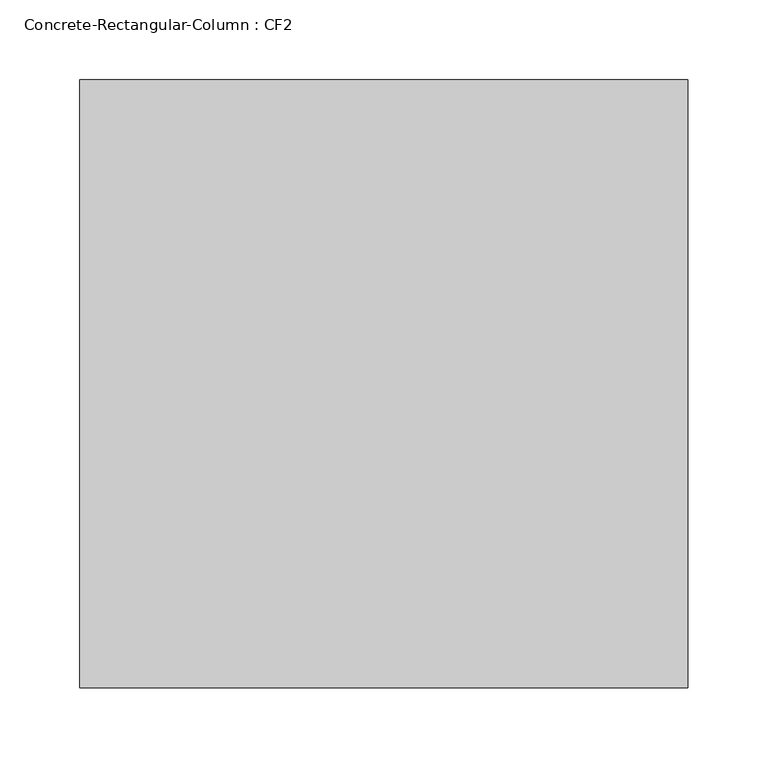
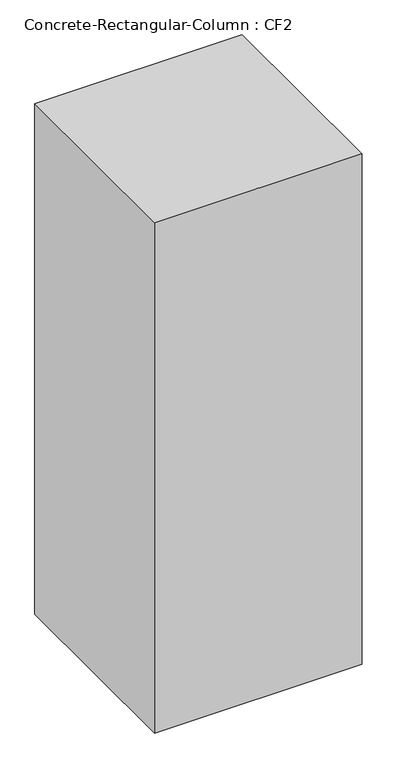
"""IFC4 building model written with IfcOpenShell, lengths in millimetres: column geometry, Concrete-Rectangular-Column : CF2."""

from ifc_helpers import new_model, si_unit, origin, origin_with_axes, place, context, project, spatial, polyline, outline, extrude, source, transform, mapped, element, save


def concrete_rectangular_column_cf2_4a54b9b5(model_context):
    return source(origin(), model_context, "Body", "SweptSolid", [
        extrude(outline(polyline([(190.5, 190.5), (190.5, -190.5), (-190.5, -190.5), (-190.5, 190.5), (190.5, 190.5)])), origin_with_axes(), (0.0, 0.0, 1.0), 990.6),
    ])


if __name__ == "__main__":
    model = new_model("IFC4")
    model_context = context("Model", 3, world=origin())
    ifc_project = project(units=[si_unit("LENGTHUNIT", "METRE", prefix="MILLI")], contexts=[model_context])
    site = spatial("IfcSite", under=ifc_project)
    building = spatial("IfcBuilding", under=site)
    placement = place(None, origin())
    concrete_rectangular_column_cf2_shape = concrete_rectangular_column_cf2_4a54b9b5(model_context)
    element("IfcColumn", 1, ObjectType="Concrete-Rectangular-Column : CF2", at=placement, inside=building, context=model_context, shape_type="MappedRepresentation", body=[
        mapped(concrete_rectangular_column_cf2_shape, transform((0.0, 0.0, 0.0), x_axis=(1.0, 0.0, 0.0), y_axis=(0.0, 1.0, 0.0), z_axis=(0.0, 0.0, 1.0))),
    ])
    save(model, "model.ifc")

# Revit data of these elements
# Type "Concrete-Rectangular-Column : CF2"
#   b = 381 mm
#   h = 381 mm
#   Structural Material [instance default] = Concrete, Cast-in-Place gray
# Element 1 (IfcColumn, "Concrete-Rectangular-Column : CF2")
#   Materials on its faces: "Concrete, Cast-in-Place gray"
# Materials
#   "Concrete, Cast-in-Place gray": class "Concrete", colour RGB 192 192 192, transparency 0, Description = "Cast-in-place concrete", Cost = 0
